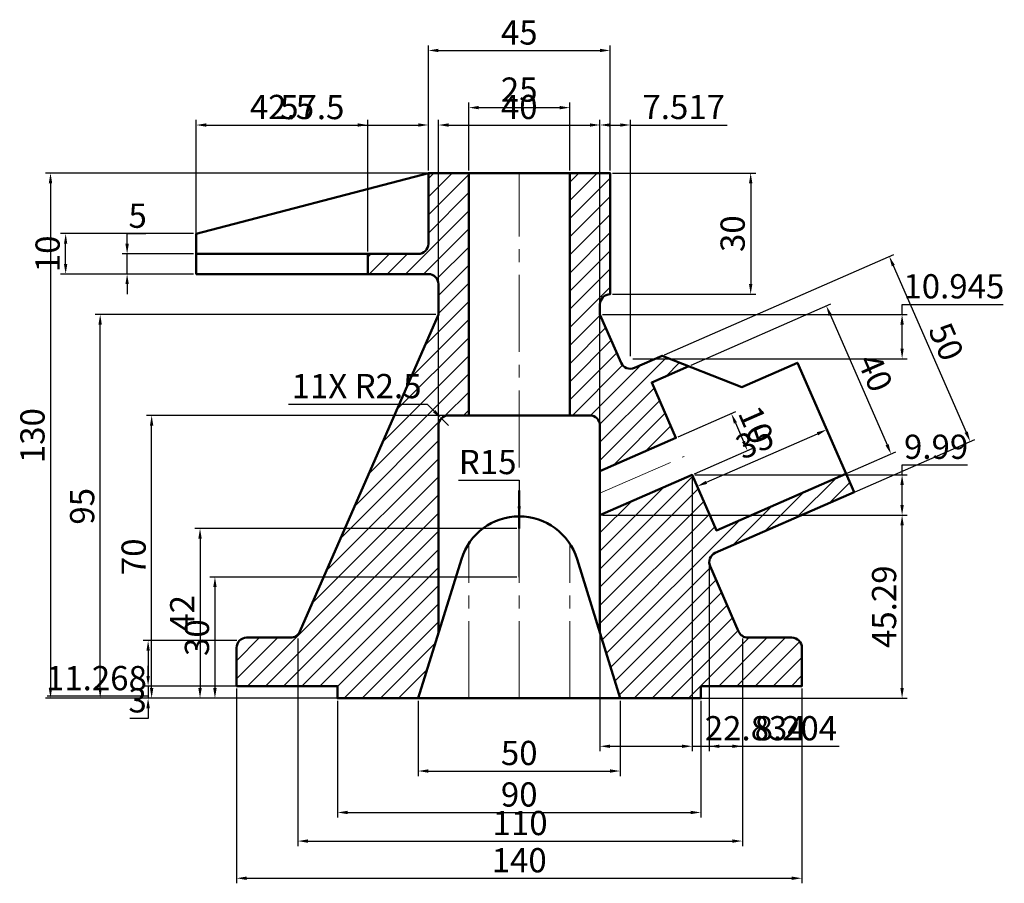
# Model space of a CAD drawing. Units: millimetres. Extents: x 76 to 320, y 39 to 253.
import ezdxf

# ---------------------------------------------------------------- set-up
doc = ezdxf.new("R2010")
doc.units = ezdxf.units.MM
doc.linetypes.add('CENTER2', pattern=[28.575, 19.05, -3.175, 3.175, -3.175])
for name, color, linetype, lineweight in [('M-CNTR', 4, 'CENTER2', 18), ('M-DIMS', 2, 'Continuous', 25), ('M-HATC', 8, 'Continuous', 18), ('M-OUTL', 7, 'Continuous', 50)]:
    doc.layers.add(name, color=color, linetype=linetype, lineweight=lineweight)
doc.styles.get("Standard").update_dxf_attribs({"font": 'arial.ttf'})
doc.dimstyles.new('ISO-25', dxfattribs={"dimtxt": 6, "dimasz": 2.5, "dimexe": 1.25, "dimexo": 0.625, "dimtad": 1, "dimtoh": 1, "dimdec": 0, "dimtxsty": 'Standard', "dimcen": 2.5, "dimadec": 0, "dimazin": 0, "dimtfac": 1, "dimtdec": 0, "dimtmove": 0, "dimatfit": 3, "dimfxl": 1, "dimarcsym": 0})

# ---------------------------------------------------------------- blocks, each defined once
blk = doc.blocks.new('*D1')
at = {"layer": 'Defpoints', "color": 0, "transparency": 16777216}
for p in [(235.21, 169.38), (311.5, 148.18), (255.25, 123.57)]:
    blk.add_point(p, dxfattribs=at)
at = {"layer": 'M-DIMS', "color": 0, "lineweight": -2, "transparency": 16777216}
for p, q in [((235.78, 169.63), (292.6, 194.49)), ((292.46, 191.7), (310.5, 150.47)), ((255.82, 123.82), (312.64, 148.68))]:
    blk.add_line(p, q, dxfattribs=at)
at = {"layer": 'M-DIMS', "color": 0, "transparency": 16777216}
for points in [[(292.84, 191.86), (292.08, 191.53), (291.46, 193.99)], [(310.88, 150.64), (310.11, 150.3), (311.5, 148.18)]]:
    blk.add_solid(points, dxfattribs=at)
at = {"layer": 'M-DIMS', "color": 0, "transparency": 16777216, "insert": (304.86, 172.56), "char_height": 6, "attachment_point": 5, "rotation": 293.6294}
blk.add_mtext('50', dxfattribs=at)
blk = doc.blocks.new('*D2')
at = {"layer": 'Defpoints', "color": 0, "transparency": 16777216}
for p in [(241.8, 166.8), (291.91, 145.07), (257.83, 130.16)]:
    blk.add_point(p, dxfattribs=at)
at = {"layer": 'M-DIMS', "color": 0, "lineweight": -2, "transparency": 16777216}
for p, q in [((242.37, 167.05), (277.02, 182.21)), ((276.88, 179.42), (290.91, 147.36)), ((258.4, 130.41), (293.05, 145.57))]:
    blk.add_line(p, q, dxfattribs=at)
at = {"layer": 'M-DIMS', "color": 0, "transparency": 16777216}
for points in [[(277.26, 179.59), (276.5, 179.25), (275.88, 181.71)], [(291.29, 147.52), (290.52, 147.19), (291.91, 145.07)]]:
    blk.add_solid(points, dxfattribs=at)
at = {"layer": 'M-DIMS', "color": 0, "transparency": 16777216, "insert": (287.27, 164.87), "char_height": 6, "attachment_point": 5, "rotation": 293.6294}
blk.add_mtext('40', dxfattribs=at)
blk = doc.blocks.new('*D3')
at = {"layer": 'Defpoints', "color": 0, "transparency": 16777216}
for p in [(238.65, 149.05), (256.36, 145.89), (242.65, 139.89)]:
    blk.add_point(p, dxfattribs=at)
at = {"layer": 'M-DIMS', "color": 0, "lineweight": -2, "transparency": 16777216}
for p, q in [((239.22, 149.3), (253.5, 155.55)), ((253.36, 152.76), (255.36, 148.18)), ((243.23, 140.14), (257.51, 146.39))]:
    blk.add_line(p, q, dxfattribs=at)
at = {"layer": 'M-DIMS', "color": 0, "transparency": 16777216}
for points in [[(253.74, 152.93), (252.98, 152.59), (252.36, 155.05)], [(255.74, 148.34), (254.98, 148.01), (256.36, 145.89)]]:
    blk.add_solid(points, dxfattribs=at)
at = {"layer": 'M-DIMS', "color": 0, "transparency": 16777216, "insert": (257.74, 151.95), "char_height": 6, "attachment_point": 5, "rotation": 293.6294}
blk.add_mtext('10', dxfattribs=at)
blk = doc.blocks.new('*D4')
at = {"layer": 'Defpoints', "color": 0, "transparency": 16777216}
for p in [(199.82, 214.61), (83.75, 84.61), (199.82, 84.61)]:
    blk.add_point(p, dxfattribs=at)
at = {"layer": 'M-DIMS', "color": 0, "lineweight": -2, "transparency": 16777216}
for p, q in [((199.2, 214.61), (82.5, 214.61)), ((83.75, 212.11), (83.75, 87.11)), ((199.2, 84.61), (82.5, 84.61))]:
    blk.add_line(p, q, dxfattribs=at)
at = {"layer": 'M-DIMS', "color": 0, "transparency": 16777216}
for points in [[(83.33, 212.11), (84.16, 212.11), (83.75, 214.61)], [(83.33, 87.11), (84.16, 87.11), (83.75, 84.61)]]:
    blk.add_solid(points, dxfattribs=at)
at = {"layer": 'M-DIMS', "color": 0, "transparency": 16777216, "insert": (80.06, 149.61), "char_height": 6, "attachment_point": 5, "rotation": 90}
blk.add_mtext('130', dxfattribs=at)
blk = doc.blocks.new('*D5')
at = {"layer": 'Defpoints', "color": 0, "transparency": 16777216}
for p in [(222.32, 214.61), (222.32, 184.61), (257.14, 184.61)]:
    blk.add_point(p, dxfattribs=at)
at = {"layer": 'M-DIMS', "color": 0, "lineweight": -2, "transparency": 16777216}
for p, q in [((222.95, 214.61), (258.39, 214.61)), ((257.14, 212.11), (257.14, 187.11)), ((222.95, 184.61), (258.39, 184.61))]:
    blk.add_line(p, q, dxfattribs=at)
at = {"layer": 'M-DIMS', "color": 0, "transparency": 16777216}
for points in [[(256.73, 212.11), (257.56, 212.11), (257.14, 214.61)], [(256.73, 187.11), (257.56, 187.11), (257.14, 184.61)]]:
    blk.add_solid(points, dxfattribs=at)
at = {"layer": 'M-DIMS', "color": 0, "transparency": 16777216, "insert": (253.45, 199.61), "char_height": 6, "attachment_point": 5, "rotation": 90}
blk.add_mtext('30', dxfattribs=at)
blk = doc.blocks.new('*D6')
at = {"layer": 'Defpoints', "color": 0, "transparency": 16777216}
for p in [(96.05, 179.61), (179.82, 179.61), (199.82, 84.61)]:
    blk.add_point(p, dxfattribs=at)
at = {"layer": 'M-DIMS', "color": 0, "lineweight": -2, "transparency": 16777216}
for p, q in [((179.2, 179.61), (94.8, 179.61)), ((96.05, 87.11), (96.05, 177.11)), ((199.2, 84.61), (94.8, 84.61))]:
    blk.add_line(p, q, dxfattribs=at)
at = {"layer": 'M-DIMS', "color": 0, "transparency": 16777216}
for points in [[(95.63, 177.11), (96.46, 177.11), (96.05, 179.61)], [(95.63, 87.11), (96.46, 87.11), (96.05, 84.61)]]:
    blk.add_solid(points, dxfattribs=at)
at = {"layer": 'M-DIMS', "color": 0, "transparency": 16777216, "insert": (92.36, 132.11), "char_height": 6, "attachment_point": 5, "rotation": 90}
blk.add_mtext('95', dxfattribs=at)
blk = doc.blocks.new('*D7')
at = {"layer": 'Defpoints', "color": 0, "transparency": 16777216}
for p in [(108.8, 154.61), (199.82, 154.61), (199.82, 84.61)]:
    blk.add_point(p, dxfattribs=at)
at = {"layer": 'M-DIMS', "color": 0, "lineweight": -2, "transparency": 16777216}
for p, q in [((199.2, 154.61), (107.55, 154.61)), ((108.8, 87.11), (108.8, 152.11)), ((199.2, 84.61), (107.55, 84.61))]:
    blk.add_line(p, q, dxfattribs=at)
at = {"layer": 'M-DIMS', "color": 0, "transparency": 16777216}
for points in [[(108.38, 152.11), (109.21, 152.11), (108.8, 154.61)], [(108.38, 87.11), (109.21, 87.11), (108.8, 84.61)]]:
    blk.add_solid(points, dxfattribs=at)
at = {"layer": 'M-DIMS', "color": 0, "transparency": 16777216, "insert": (105.11, 119.61), "char_height": 6, "attachment_point": 5, "rotation": 90}
blk.add_mtext('70', dxfattribs=at)
blk = doc.blocks.new('*D8')
at = {"layer": 'Defpoints', "color": 0, "transparency": 16777216}
for p in [(222.32, 244.97), (177.32, 214.61), (222.32, 214.61)]:
    blk.add_point(p, dxfattribs=at)
at = {"layer": 'M-DIMS', "color": 0, "lineweight": -2, "transparency": 16777216}
for p, q in [((177.32, 215.23), (177.32, 246.22)), ((179.82, 244.97), (219.82, 244.97)), ((222.32, 215.23), (222.32, 246.22))]:
    blk.add_line(p, q, dxfattribs=at)
at = {"layer": 'M-DIMS', "color": 0, "transparency": 16777216}
for points in [[(179.82, 245.38), (179.82, 244.55), (177.32, 244.97)], [(219.82, 245.38), (219.82, 244.55), (222.32, 244.97)]]:
    blk.add_solid(points, dxfattribs=at)
at = {"layer": 'M-DIMS', "color": 0, "transparency": 16777216, "insert": (199.82, 248.64), "char_height": 6, "attachment_point": 5}
blk.add_mtext('45', dxfattribs=at)
blk = doc.blocks.new('*D9')
at = {"layer": 'Defpoints', "color": 0, "transparency": 16777216}
for p in [(212.32, 230.81), (187.32, 214.61), (212.32, 214.61)]:
    blk.add_point(p, dxfattribs=at)
at = {"layer": 'M-DIMS', "color": 0, "lineweight": -2, "transparency": 16777216}
for p, q in [((187.32, 215.23), (187.32, 232.06)), ((212.32, 215.23), (212.32, 232.06)), ((189.82, 230.81), (209.82, 230.81))]:
    blk.add_line(p, q, dxfattribs=at)
at = {"layer": 'M-DIMS', "color": 0, "transparency": 16777216}
for points in [[(189.82, 231.23), (189.82, 230.39), (187.32, 230.81)], [(209.82, 231.23), (209.82, 230.39), (212.32, 230.81)]]:
    blk.add_solid(points, dxfattribs=at)
at = {"layer": 'M-DIMS', "color": 0, "transparency": 16777216, "insert": (199.82, 234.5), "char_height": 6, "attachment_point": 5}
blk.add_mtext('25', dxfattribs=at)
blk = doc.blocks.new('*D10')
at = {"layer": 'Defpoints', "color": 0, "transparency": 16777216}
for p in [(87.5, 199.61), (119.82, 199.61), (119.82, 189.61)]:
    blk.add_point(p, dxfattribs=at)
at = {"layer": 'M-DIMS', "color": 0, "lineweight": -2, "transparency": 16777216}
for p, q in [((119.2, 199.61), (86.25, 199.61)), ((87.5, 192.11), (87.5, 197.11)), ((119.2, 189.61), (86.25, 189.61))]:
    blk.add_line(p, q, dxfattribs=at)
at = {"layer": 'M-DIMS', "color": 0, "transparency": 16777216}
for points in [[(87.08, 197.11), (87.91, 197.11), (87.5, 199.61)], [(87.08, 192.11), (87.91, 192.11), (87.5, 189.61)]]:
    blk.add_solid(points, dxfattribs=at)
at = {"layer": 'M-DIMS', "color": 0, "transparency": 16777216, "insert": (83.81, 194.61), "char_height": 6, "attachment_point": 5, "rotation": 90}
blk.add_mtext('10', dxfattribs=at)
blk = doc.blocks.new('*D11')
at = {"layer": 'Defpoints', "color": 0, "transparency": 16777216}
for p in [(102.72, 194.61), (119.82, 194.61), (119.82, 189.61)]:
    blk.add_point(p, dxfattribs=at)
at = {"layer": 'M-DIMS', "color": 0, "lineweight": -2, "transparency": 16777216}
for p, q in [((102.72, 197.11), (102.72, 199.61)), ((102.72, 199.61), (107.32, 199.61)), ((119.2, 194.61), (101.47, 194.61)), ((102.72, 189.61), (102.72, 194.61)), ((119.2, 189.61), (101.47, 189.61)), ((102.72, 187.11), (102.72, 184.61))]:
    blk.add_line(p, q, dxfattribs=at)
at = {"layer": 'M-DIMS', "color": 0, "transparency": 16777216}
for points in [[(102.3, 197.11), (103.14, 197.11), (102.72, 194.61)], [(102.3, 187.11), (103.14, 187.11), (102.72, 189.61)]]:
    blk.add_solid(points, dxfattribs=at)
at = {"layer": 'M-DIMS', "color": 0, "transparency": 16777216, "insert": (105.33, 203.28), "char_height": 6, "attachment_point": 5}
blk.add_mtext('5', dxfattribs=at)
blk = doc.blocks.new('*D12')
at = {"layer": 'Defpoints', "color": 0, "transparency": 16777216}
for p in [(129.82, 87.61), (269.82, 87.61), (269.82, 40.03)]:
    blk.add_point(p, dxfattribs=at)
at = {"layer": 'M-DIMS', "color": 0, "lineweight": -2, "transparency": 16777216}
for p, q in [((129.82, 86.98), (129.82, 38.78)), ((269.82, 86.98), (269.82, 38.78)), ((132.32, 40.03), (267.32, 40.03))]:
    blk.add_line(p, q, dxfattribs=at)
at = {"layer": 'M-DIMS', "color": 0, "transparency": 16777216}
for points in [[(132.32, 40.45), (132.32, 39.62), (129.82, 40.03)], [(267.32, 40.45), (267.32, 39.62), (269.82, 40.03)]]:
    blk.add_solid(points, dxfattribs=at)
at = {"layer": 'M-DIMS', "color": 0, "transparency": 16777216, "insert": (199.82, 43.72), "char_height": 6, "attachment_point": 5}
blk.add_mtext('140', dxfattribs=at)
blk = doc.blocks.new('*D13')
at = {"layer": 'Defpoints', "color": 0, "transparency": 16777216}
for p in [(174.82, 84.61), (224.82, 84.61), (224.82, 66.58)]:
    blk.add_point(p, dxfattribs=at)
at = {"layer": 'M-DIMS', "color": 0, "lineweight": -2, "transparency": 16777216}
for p, q in [((174.82, 83.98), (174.82, 65.33)), ((224.82, 83.98), (224.82, 65.33)), ((177.32, 66.58), (222.32, 66.58))]:
    blk.add_line(p, q, dxfattribs=at)
at = {"layer": 'M-DIMS', "color": 0, "transparency": 16777216}
for points in [[(177.32, 67), (177.32, 66.16), (174.82, 66.58)], [(222.32, 67), (222.32, 66.16), (224.82, 66.58)]]:
    blk.add_solid(points, dxfattribs=at)
at = {"layer": 'M-DIMS', "color": 0, "transparency": 16777216, "insert": (199.82, 70.27), "char_height": 6, "attachment_point": 5}
blk.add_mtext('50', dxfattribs=at)
blk = doc.blocks.new('*D14')
at = {"layer": 'Defpoints', "color": 0, "transparency": 16777216}
for p in [(154.82, 84.61), (244.82, 84.61), (244.82, 56.32)]:
    blk.add_point(p, dxfattribs=at)
at = {"layer": 'M-DIMS', "color": 0, "lineweight": -2, "transparency": 16777216}
for p, q in [((154.82, 83.98), (154.82, 55.07)), ((244.82, 83.98), (244.82, 55.07)), ((157.32, 56.32), (242.32, 56.32))]:
    blk.add_line(p, q, dxfattribs=at)
at = {"layer": 'M-DIMS', "color": 0, "transparency": 16777216}
for points in [[(157.32, 56.73), (157.32, 55.9), (154.82, 56.32)], [(242.32, 56.73), (242.32, 55.9), (244.82, 56.32)]]:
    blk.add_solid(points, dxfattribs=at)
at = {"layer": 'M-DIMS', "color": 0, "transparency": 16777216, "insert": (199.82, 60), "char_height": 6, "attachment_point": 5}
blk.add_mtext('90', dxfattribs=at)
blk = doc.blocks.new('*D15')
at = {"layer": 'Defpoints', "color": 0, "transparency": 16777216}
for p in [(144.99, 99.99), (255.09, 100.01), (255.09, 49.24)]:
    blk.add_point(p, dxfattribs=at)
at = {"layer": 'M-DIMS', "color": 0, "lineweight": -2, "transparency": 16777216}
for p, q in [((144.99, 99.37), (144.99, 47.99)), ((255.09, 99.39), (255.09, 47.99)), ((147.49, 49.24), (252.59, 49.24))]:
    blk.add_line(p, q, dxfattribs=at)
at = {"layer": 'M-DIMS', "color": 0, "transparency": 16777216}
for points in [[(147.49, 49.65), (147.49, 48.82), (144.99, 49.24)], [(252.59, 49.65), (252.59, 48.82), (255.09, 49.24)]]:
    blk.add_solid(points, dxfattribs=at)
at = {"layer": 'M-DIMS', "color": 0, "transparency": 16777216, "insert": (200.04, 52.93), "char_height": 6, "attachment_point": 5}
blk.add_mtext('110', dxfattribs=at)
blk = doc.blocks.new('*D16')
at = {"layer": 'Defpoints', "color": 0, "transparency": 16777216}
for p in [(199.82, 114.61), (124.47, 84.61), (199.82, 84.61)]:
    blk.add_point(p, dxfattribs=at)
at = {"layer": 'M-DIMS', "color": 0, "lineweight": -2, "transparency": 16777216}
for p, q in [((199.2, 114.61), (123.22, 114.61)), ((124.47, 112.11), (124.47, 87.11)), ((199.2, 84.61), (123.22, 84.61))]:
    blk.add_line(p, q, dxfattribs=at)
at = {"layer": 'M-DIMS', "color": 0, "transparency": 16777216}
for points in [[(124.05, 112.11), (124.89, 112.11), (124.47, 114.61)], [(124.05, 87.11), (124.89, 87.11), (124.47, 84.61)]]:
    blk.add_solid(points, dxfattribs=at)
at = {"layer": 'M-DIMS', "color": 0, "transparency": 16777216, "insert": (120.78, 99.61), "char_height": 6, "attachment_point": 5, "rotation": 90}
blk.add_mtext('30', dxfattribs=at)
blk = doc.blocks.new('*D17')
at = {"layer": 'Defpoints', "color": 0, "transparency": 16777216}
for p in [(199.82, 126.61), (120.78, 84.61), (199.82, 84.61)]:
    blk.add_point(p, dxfattribs=at)
at = {"layer": 'M-DIMS', "color": 0, "lineweight": -2, "transparency": 16777216}
for p, q in [((199.2, 126.61), (119.53, 126.61)), ((120.78, 124.11), (120.78, 87.11)), ((199.2, 84.61), (119.53, 84.61))]:
    blk.add_line(p, q, dxfattribs=at)
at = {"layer": 'M-DIMS', "color": 0, "transparency": 16777216}
for points in [[(120.36, 124.11), (121.2, 124.11), (120.78, 126.61)], [(120.36, 87.11), (121.2, 87.11), (120.78, 84.61)]]:
    blk.add_solid(points, dxfattribs=at)
at = {"layer": 'M-DIMS', "color": 0, "transparency": 16777216, "insert": (117.14, 105.61), "char_height": 6, "attachment_point": 5, "rotation": 90}
blk.add_mtext('42', dxfattribs=at)
blk = doc.blocks.new('*D18')
at = {"layer": 'Defpoints', "color": 0, "transparency": 16777216}
for p in [(177.32, 226.51), (177.32, 214.61), (119.82, 199.61)]:
    blk.add_point(p, dxfattribs=at)
at = {"layer": 'M-DIMS', "color": 0, "lineweight": -2, "transparency": 16777216}
for p, q in [((119.82, 200.23), (119.82, 227.76)), ((177.32, 215.23), (177.32, 227.76)), ((122.32, 226.51), (174.82, 226.51))]:
    blk.add_line(p, q, dxfattribs=at)
at = {"layer": 'M-DIMS', "color": 0, "transparency": 16777216}
for points in [[(122.32, 226.92), (122.32, 226.09), (119.82, 226.51)], [(174.82, 226.92), (174.82, 226.09), (177.32, 226.51)]]:
    blk.add_solid(points, dxfattribs=at)
at = {"layer": 'M-DIMS', "color": 0, "transparency": 16777216, "insert": (148.57, 230.18), "char_height": 6, "attachment_point": 5}
blk.add_mtext('57.5', dxfattribs=at)
blk = doc.blocks.new('*D19')
at = {"layer": 'Defpoints', "color": 0, "transparency": 16777216}
for p in [(162.32, 226.51), (162.32, 194.61), (119.82, 189.61)]:
    blk.add_point(p, dxfattribs=at)
at = {"layer": 'M-DIMS', "color": 0, "lineweight": -2, "transparency": 16777216}
for p, q in [((119.82, 190.23), (119.82, 227.76)), ((162.32, 195.23), (162.32, 227.76)), ((122.32, 226.51), (159.82, 226.51))]:
    blk.add_line(p, q, dxfattribs=at)
at = {"layer": 'M-DIMS', "color": 0, "transparency": 16777216}
for points in [[(122.32, 226.92), (122.32, 226.09), (119.82, 226.51)], [(159.82, 226.92), (159.82, 226.09), (162.32, 226.51)]]:
    blk.add_solid(points, dxfattribs=at)
at = {"layer": 'M-DIMS', "color": 0, "transparency": 16777216, "insert": (141.07, 230.2), "char_height": 6, "attachment_point": 5}
blk.add_mtext('42.5', dxfattribs=at)
blk = doc.blocks.new('*D20')
at = {"layer": 'Defpoints', "color": 0, "transparency": 16777216}
for p in [(130.55, 98.87), (107.92, 87.61), (129.82, 87.61)]:
    blk.add_point(p, dxfattribs=at)
at = {"layer": 'M-DIMS', "color": 0, "lineweight": -2, "transparency": 16777216}
for p, q in [((129.93, 98.87), (106.67, 98.87)), ((107.92, 96.37), (107.92, 90.11)), ((129.2, 87.61), (106.67, 87.61)), ((107.92, 87.61), (107.92, 85.11)), ((107.92, 85.11), (82.94, 85.11))]:
    blk.add_line(p, q, dxfattribs=at)
at = {"layer": 'M-DIMS', "color": 0, "transparency": 16777216}
for points in [[(107.5, 96.37), (108.34, 96.37), (107.92, 98.87)], [(107.5, 90.11), (108.34, 90.11), (107.92, 87.61)]]:
    blk.add_solid(points, dxfattribs=at)
at = {"layer": 'M-DIMS', "color": 0, "transparency": 16777216, "insert": (95.12, 88.8), "char_height": 6, "attachment_point": 5}
blk.add_mtext('11.268', dxfattribs=at)
blk = doc.blocks.new('*D21')
at = {"layer": 'Defpoints', "color": 0, "transparency": 16777216}
for p in [(154.82, 87.61), (107.92, 84.61), (154.82, 84.61)]:
    blk.add_point(p, dxfattribs=at)
at = {"layer": 'M-DIMS', "color": 0, "lineweight": -2, "transparency": 16777216}
for p, q in [((107.92, 90.11), (107.92, 92.61)), ((154.2, 87.61), (106.67, 87.61)), ((107.92, 87.61), (107.92, 84.61)), ((154.2, 84.61), (106.67, 84.61)), ((107.92, 82.11), (107.92, 79.61)), ((107.92, 79.61), (103.37, 79.61))]:
    blk.add_line(p, q, dxfattribs=at)
at = {"layer": 'M-DIMS', "color": 0, "transparency": 16777216}
for points in [[(107.5, 90.11), (108.34, 90.11), (107.92, 87.61)], [(107.5, 82.11), (108.34, 82.11), (107.92, 84.61)]]:
    blk.add_solid(points, dxfattribs=at)
at = {"layer": 'M-DIMS', "color": 0, "transparency": 16777216, "insert": (105.33, 83.3), "char_height": 6, "attachment_point": 5}
blk.add_mtext('3', dxfattribs=at)
blk = doc.blocks.new('*D22')
at = {"layer": 'Defpoints', "color": 0, "transparency": 16777216}
for p in [(219.82, 226.51), (179.82, 152.11), (219.82, 152.11)]:
    blk.add_point(p, dxfattribs=at)
at = {"layer": 'M-DIMS', "color": 0, "lineweight": -2, "transparency": 16777216}
for p, q in [((179.82, 152.73), (179.82, 227.76)), ((219.82, 152.73), (219.82, 227.76)), ((182.32, 226.51), (217.32, 226.51))]:
    blk.add_line(p, q, dxfattribs=at)
at = {"layer": 'M-DIMS', "color": 0, "transparency": 16777216}
for points in [[(182.32, 226.92), (182.32, 226.09), (179.82, 226.51)], [(217.32, 226.92), (217.32, 226.09), (219.82, 226.51)]]:
    blk.add_solid(points, dxfattribs=at)
at = {"layer": 'M-DIMS', "color": 0, "transparency": 16777216, "insert": (199.82, 230.2), "char_height": 6, "attachment_point": 5}
blk.add_mtext('40', dxfattribs=at)
blk = doc.blocks.new('*D23')
at = {"layer": 'Defpoints', "color": 0, "transparency": 16777216}
for p in [(227.34, 226.51), (219.82, 179.61), (227.34, 168.66)]:
    blk.add_point(p, dxfattribs=at)
at = {"layer": 'M-DIMS', "color": 0, "lineweight": -2, "transparency": 16777216}
for p, q in [((219.82, 180.23), (219.82, 227.76)), ((227.34, 169.29), (227.34, 227.76)), ((222.32, 226.51), (224.84, 226.51)), ((227.34, 226.51), (251.29, 226.51))]:
    blk.add_line(p, q, dxfattribs=at)
at = {"layer": 'M-DIMS', "color": 0, "transparency": 16777216}
for points in [[(222.32, 226.92), (222.32, 226.09), (219.82, 226.51)], [(224.84, 226.92), (224.84, 226.09), (227.34, 226.51)]]:
    blk.add_solid(points, dxfattribs=at)
at = {"layer": 'M-DIMS', "color": 0, "transparency": 16777216, "insert": (240.56, 230.2), "char_height": 6, "attachment_point": 5}
blk.add_mtext('7.517', dxfattribs=at)
blk = doc.blocks.new('*D24')
at = {"layer": 'Defpoints', "color": 0, "transparency": 16777216}
for p in [(219.82, 179.61), (294.64, 179.61), (227.34, 168.66)]:
    blk.add_point(p, dxfattribs=at)
at = {"layer": 'M-DIMS', "color": 0, "lineweight": -2, "transparency": 16777216}
for p, q in [((294.64, 179.61), (294.64, 182.11)), ((294.64, 182.11), (319.65, 182.11)), ((220.45, 179.61), (295.89, 179.61)), ((294.64, 171.16), (294.64, 177.11)), ((227.96, 168.66), (295.89, 168.66))]:
    blk.add_line(p, q, dxfattribs=at)
at = {"layer": 'M-DIMS', "color": 0, "transparency": 16777216}
for points in [[(294.22, 177.11), (295.05, 177.11), (294.64, 179.61)], [(294.22, 171.16), (295.05, 171.16), (294.64, 168.66)]]:
    blk.add_solid(points, dxfattribs=at)
at = {"layer": 'M-DIMS', "color": 0, "transparency": 16777216, "insert": (307.46, 185.8), "char_height": 6, "attachment_point": 5}
blk.add_mtext('10.945', dxfattribs=at)
blk = doc.blocks.new('*D25')
at = {"layer": 'Defpoints', "color": 0, "transparency": 16777216}
for p in [(242.65, 139.89), (219.82, 129.9), (242.65, 72.71)]:
    blk.add_point(p, dxfattribs=at)
at = {"layer": 'M-DIMS', "color": 0, "lineweight": -2, "transparency": 16777216}
for p, q in [((242.65, 139.26), (242.65, 71.46)), ((219.82, 129.27), (219.82, 71.46)), ((222.32, 72.71), (240.15, 72.71)), ((242.65, 72.71), (271.39, 72.71))]:
    blk.add_line(p, q, dxfattribs=at)
at = {"layer": 'M-DIMS', "color": 0, "transparency": 16777216}
for points in [[(222.32, 73.12), (222.32, 72.29), (219.82, 72.71)], [(240.15, 73.12), (240.15, 72.29), (242.65, 72.71)]]:
    blk.add_solid(points, dxfattribs=at)
at = {"layer": 'M-DIMS', "color": 0, "transparency": 16777216, "insert": (258.27, 76.4), "char_height": 6, "attachment_point": 5}
blk.add_mtext('22.834', dxfattribs=at)
blk = doc.blocks.new('*D26')
at = {"layer": 'Defpoints', "color": 0, "transparency": 16777216}
for p in [(242.65, 139.89), (294.64, 139.89), (219.82, 129.9)]:
    blk.add_point(p, dxfattribs=at)
at = {"layer": 'M-DIMS', "color": 0, "lineweight": -2, "transparency": 16777216}
for p, q in [((294.64, 139.89), (294.64, 142.39)), ((294.64, 142.39), (310.86, 142.39)), ((243.28, 139.89), (295.89, 139.89)), ((294.64, 132.4), (294.64, 137.39)), ((220.45, 129.9), (295.89, 129.9))]:
    blk.add_line(p, q, dxfattribs=at)
at = {"layer": 'M-DIMS', "color": 0, "transparency": 16777216}
for points in [[(294.22, 137.39), (295.05, 137.39), (294.64, 139.89)], [(294.22, 132.4), (295.05, 132.4), (294.64, 129.9)]]:
    blk.add_solid(points, dxfattribs=at)
at = {"layer": 'M-DIMS', "color": 0, "transparency": 16777216, "insert": (303.06, 146.08), "char_height": 6, "attachment_point": 5}
blk.add_mtext('9.99', dxfattribs=at)
blk = doc.blocks.new('*D27')
at = {"layer": 'Defpoints', "color": 0, "transparency": 16777216}
for p in [(219.82, 129.9), (294.64, 129.9), (224.82, 84.61)]:
    blk.add_point(p, dxfattribs=at)
at = {"layer": 'M-DIMS', "color": 0, "lineweight": -2, "transparency": 16777216}
for p, q in [((220.45, 129.9), (295.89, 129.9)), ((294.64, 87.11), (294.64, 127.4)), ((225.45, 84.61), (295.89, 84.61))]:
    blk.add_line(p, q, dxfattribs=at)
at = {"layer": 'M-DIMS', "color": 0, "transparency": 16777216}
for points in [[(294.22, 127.4), (295.05, 127.4), (294.64, 129.9)], [(294.22, 87.11), (295.05, 87.11), (294.64, 84.61)]]:
    blk.add_solid(points, dxfattribs=at)
at = {"layer": 'M-DIMS', "color": 0, "transparency": 16777216, "insert": (290.95, 107.25), "char_height": 6, "attachment_point": 5, "rotation": 90}
blk.add_mtext('45.29', dxfattribs=at)
blk = doc.blocks.new('*D28')
at = {"layer": 'Defpoints', "color": 0, "transparency": 16777216}
for p in [(246.88, 118.22), (255.09, 100.01), (255.09, 72.71)]:
    blk.add_point(p, dxfattribs=at)
at = {"layer": 'M-DIMS', "color": 0, "lineweight": -2, "transparency": 16777216}
for p, q in [((246.88, 117.6), (246.88, 71.46)), ((255.09, 99.39), (255.09, 71.46)), ((249.38, 72.71), (252.59, 72.71)), ((255.09, 72.71), (279.07, 72.71))]:
    blk.add_line(p, q, dxfattribs=at)
at = {"layer": 'M-DIMS', "color": 0, "transparency": 16777216}
for points in [[(249.38, 73.12), (249.38, 72.29), (246.88, 72.71)], [(252.59, 73.12), (252.59, 72.29), (255.09, 72.71)]]:
    blk.add_solid(points, dxfattribs=at)
at = {"layer": 'M-DIMS', "color": 0, "transparency": 16777216, "insert": (268.33, 76.4), "char_height": 6, "attachment_point": 5}
blk.add_mtext('8.204', dxfattribs=at)
blk = doc.blocks.new('*D29')
at = {"layer": 'Defpoints', "color": 0, "transparency": 16777216}
for p in [(275.96, 151.08), (280.73, 140.18), (248.67, 126.15)]:
    blk.add_point(p, dxfattribs=at)
at = {"layer": 'M-DIMS', "color": 0, "lineweight": -2, "transparency": 16777216}
for p, q in [((280.48, 140.75), (275.46, 152.22)), ((246.19, 138.05), (273.67, 150.08)), ((248.42, 126.72), (243.4, 138.19))]:
    blk.add_line(p, q, dxfattribs=at)
at = {"layer": 'M-DIMS', "color": 0, "transparency": 16777216}
for points in [[(273.51, 150.46), (273.84, 149.69), (275.96, 151.08)], [(246.02, 138.43), (246.35, 137.67), (243.9, 137.05)]]:
    blk.add_solid(points, dxfattribs=at)
at = {"layer": 'M-DIMS', "color": 0, "transparency": 16777216, "insert": (258.45, 147.44), "char_height": 6, "attachment_point": 5, "rotation": 23.6294}
blk.add_mtext('35', dxfattribs=at)
blk = doc.blocks.new('*D30')
at = {"layer": 'Defpoints', "color": 0, "transparency": 16777216}
for p in [(199.82, 129.61), (199.82, 114.61)]:
    blk.add_point(p, dxfattribs=at)
at = {"layer": 'M-DIMS', "color": 0, "lineweight": -2, "transparency": 16777216}
for p, q in [((184.81, 138.61), (199.82, 138.61)), ((199.82, 138.61), (199.82, 132.11)), ((199.82, 114.61), (199.82, 129.61))]:
    blk.add_line(p, q, dxfattribs=at)
at = {"layer": 'M-DIMS', "color": 0, "transparency": 16777216}
blk.add_solid([(200.24, 132.11), (199.4, 132.11), (199.82, 129.61)], dxfattribs=at)
at = {"layer": 'M-DIMS', "color": 0, "transparency": 16777216, "insert": (192, 142.3), "char_height": 6, "attachment_point": 5}
blk.add_mtext('R15', dxfattribs=at)
blk = doc.blocks.new('*D31')
at = {"layer": 'Defpoints', "color": 0, "transparency": 16777216}
for p in [(180.55, 153.87), (182.32, 152.11)]:
    blk.add_point(p, dxfattribs=at)
at = {"layer": 'M-DIMS', "color": 0, "lineweight": -2, "transparency": 16777216}
for p, q in [((142.69, 157.41), (177.02, 157.41)), ((177.02, 157.41), (178.79, 155.64)), ((182.32, 152.11), (180.55, 153.87))]:
    blk.add_line(p, q, dxfattribs=at)
at = {"layer": 'M-DIMS', "color": 0, "transparency": 16777216}
blk.add_solid([(179.08, 155.94), (178.49, 155.35), (180.55, 153.87)], dxfattribs=at)
at = {"layer": 'M-DIMS', "color": 0, "transparency": 16777216, "insert": (159.54, 161.1), "char_height": 6, "attachment_point": 5}
blk.add_mtext('11X R2.5', dxfattribs=at)

msp = doc.modelspace()

# ---------------------------------------------------------------- hatches: boundary and pattern name
at = {"layer": 'M-HATC'}
h = msp.add_hatch(dxfattribs=at)
h.set_pattern_fill('ANSI31', color=256)
h.paths.add_polyline_path([(179.8208, 152.1071, -0.41421356), (182.3208, 154.6071), (187.3208, 154.6071), (187.3208, 214.6071), (177.3208, 214.6071), (177.3208, 197.1071, -0.41421356), (174.8208, 194.6071), (162.3208, 194.6071), (162.3208, 189.6071), (177.3208, 189.6071, -0.41421356), (179.8208, 187.1071), (179.8208, 179.6071), (145.4762, 101.1051, -0.29797338), (143.1858, 99.6071), (132.3208, 99.6071, 0.41421356), (129.8208, 97.1071), (129.8208, 87.6071), (154.8208, 87.6071), (154.8208, 84.6071), (174.8208, 84.6071), (179.8208, 100.7425)])
h.paths.add_polyline_path([(222.3208, 184.6071), (222.3208, 214.6071), (212.3208, 214.6071), (212.3208, 154.6071), (217.3208, 154.6071, -0.41421356), (219.8208, 152.1071), (219.8208, 140.8147), (238.6467, 149.051), (232.6344, 162.7934), (241.796, 166.8016), (235.2111, 169.3783), (228.3399, 166.3721, -0.41421356), (225.0475, 167.6605), (219.8208, 179.6071), (219.8208, 182.1071, -0.41421356)])
h = msp.add_hatch(dxfattribs=at)
h.set_pattern_fill('ANSI31', color=256)
h.paths.add_polyline_path([(247.0925, 117.2718, -0.41421356), (248.3808, 120.5643), (282.7367, 135.595), (280.7326, 140.1757), (248.6671, 126.1471), (242.6549, 139.8894), (219.8208, 129.8995), (219.8208, 100.7425), (224.8208, 84.6071), (244.8208, 84.6071), (244.8208, 87.6071), (269.8208, 87.6071), (269.8208, 97.1071, 0.41421356), (267.3208, 99.6071), (256.4558, 99.6071, -0.29797338), (254.1654, 101.1051)])

# ---------------------------------------------------------------- linework, layer by layer
at = {"layer": 'M-CNTR'}
for p, q in [((199.8208, 84.6071), (199.8208, 214.6071)), ((219.8208, 135.3571), (240.6508, 144.4702)), ((187.3208, 84.6071), (187.3208, 122.8987)), ((212.3208, 84.6071), (212.3208, 122.8987))]:
    msp.add_line(p, q, dxfattribs=at)
at = {"layer": 'M-OUTL'}
for p, q in [((187.3208, 154.6071), (187.3208, 214.6071)), ((212.3208, 154.6071), (212.3208, 214.6071)), ((162.3208, 194.6071), (162.3208, 189.6071)), ((199.8208, 126.6071), (199.8208, 136.0672))]:
    msp.add_line(p, q, dxfattribs=at)
for points in [[(224.8208, 84.6071), (244.8208, 84.6071), (244.8208, 87.6071), (269.8208, 87.6071), (269.8208, 97.1071, 0.41421356), (267.3208, 99.6071), (256.4558, 99.6071, -0.29797338), (254.1654, 101.1051), (247.0925, 117.2718, -0.41421356), (248.3808, 120.5643), (282.7367, 135.595), (268.7081, 167.6605), (254.9657, 161.6482), (235.2111, 169.3783), (228.3399, 166.3721, -0.41421356), (225.0475, 167.6605), (219.8208, 179.6071), (219.8208, 182.1071, -0.41421356), (222.3208, 184.6071), (222.3208, 184.6071), (222.3208, 214.6071), (199.8208, 214.6071), (177.3208, 214.6071), (119.8208, 199.6071), (119.8208, 194.6071)], [(177.3208, 214.6071), (177.3208, 197.1071, -0.41421356), (174.8208, 194.6071), (119.8208, 194.6071), (119.8208, 189.6071), (177.3208, 189.6071, -0.41421356), (179.8208, 187.1071), (179.8208, 179.6071), (145.4762, 101.1051, -0.29797338), (143.1858, 99.6071), (132.3208, 99.6071, 0.41421356), (129.8208, 97.1071), (129.8208, 87.6071), (154.8208, 87.6071), (154.8208, 84.6071), (174.8208, 84.6071)], [(219.8208, 100.7425), (219.8208, 152.1071, 0.41421356), (217.3208, 154.6071), (182.3208, 154.6071, 0.41421356), (179.8208, 152.1071), (179.8208, 100.7425)]]:
    msp.add_lwpolyline(points, format="xyb", dxfattribs=at)
for points in [[(219.8208, 140.8147), (238.6467, 149.051), (232.6344, 162.7934), (241.796, 166.8016)], [(219.8208, 129.8995), (242.6549, 139.8894), (248.6671, 126.1471), (280.7326, 140.1757)]]:
    msp.add_lwpolyline(points, dxfattribs=at)
msp.add_lwpolyline([(185.4929, 119.047), (174.8208, 84.6071), (224.8208, 84.6071), (214.1487, 119.047, 0.73703418)], format="xyb", close=True, dxfattribs=at)

# ---------------------------------------------------------------- dimensions: what is measured, and where the dimension line sits
at = {"layer": 'M-DIMS'}
for base, p1, p2, override, picture, middle in [((222.3208, 244.9667), (177.3208, 214.6071), (222.3208, 214.6071), {"dimclrd": 0, "dimclre": 0, "dimclrt": 0}, '*D8', (199.8208, 248.6429)), ((212.3208, 230.8091), (187.3208, 214.6071), (212.3208, 214.6071), {"dimclrd": 0, "dimclre": 0, "dimclrt": 0}, '*D9', (199.8208, 234.4975)), ((162.3208, 226.5071), (119.8208, 189.6071), (162.3208, 194.6071), {"dimdec": 1, "dimlfac": 1, "dimrnd": 0, "dimzin": 0, "dimdsep": 46, "dimlunit": 2}, '*D19', (141.0708, 230.1956)), ((177.3208, 226.5071), (119.8208, 199.6071), (177.3208, 214.6071), {"dimdec": 1, "dimlfac": 1, "dimrnd": 0, "dimzin": 0, "dimdsep": 46, "dimlunit": 2}, '*D18', (148.5708, 230.1833)), ((219.8208, 226.5071), (179.8208, 152.1071), (219.8208, 152.1071), {"dimdec": 0, "dimlfac": 1, "dimrnd": 0, "dimzin": 0, "dimdsep": 46, "dimlunit": 2}, '*D22', (199.8208, 230.1956)), ((227.3379, 226.5071), (219.8208, 179.6071), (227.3379, 168.6625), {"dimdec": 3, "dimlfac": 1, "dimrnd": 0, "dimzin": 0, "dimdsep": 46, "dimlunit": 2}, '*D23', (240.5618, 230.1956)), ((242.6549, 72.7071), (219.8208, 129.8995), (242.6549, 139.8894), {"dimdec": 3, "dimlfac": 1, "dimrnd": 0, "dimzin": 0, "dimdsep": 46, "dimlunit": 2}, '*D25', (258.273, 76.3976)), ((255.0875, 72.7071), (246.8834, 118.2246), (255.0875, 100.0149), {"dimdec": 3, "dimlfac": 1, "dimrnd": 0, "dimzin": 0, "dimdsep": 46, "dimlunit": 2}, '*D28', (268.3277, 76.3956)), ((255.0875, 49.2368), (144.9892, 99.992), (255.0875, 100.0149), {"dimclrd": 0, "dimclre": 0, "dimclrt": 0}, '*D15', (200.0383, 52.9253)), ((269.8208, 40.0343), (129.8208, 87.6071), (269.8208, 87.6071), {"dimclrd": 0, "dimclre": 0, "dimclrt": 0}, '*D12', (199.8208, 43.7228)), ((244.8208, 56.3157), (154.8208, 84.6071), (244.8208, 84.6071), {"dimclrd": 0, "dimclre": 0, "dimclrt": 0}, '*D14', (199.8208, 60.0041)), ((224.8208, 66.58), (174.8208, 84.6071), (224.8208, 84.6071), {"dimclrd": 0, "dimclre": 0, "dimclrt": 0}, '*D13', (199.8208, 70.2684))]:
    dim = msp.add_linear_dim(base=base, p1=p1, p2=p2, dimstyle='ISO-25', override=override, dxfattribs=at)
    dim.commit()
    dim.dimension.update_dxf_attribs({"geometry": picture, "text_midpoint": middle})
for base, p1, p2, angle, override, picture, middle in [((83.7456, 84.6071), (199.8208, 214.6071), (199.8208, 84.6071), 90, {"dimclrd": 0, "dimclre": 0, "dimclrt": 0}, '*D4', (80.0552, 149.6071)), ((257.144, 184.6071), (222.3208, 214.6071), (222.3208, 184.6071), 90, {"dimclrd": 0, "dimclre": 0, "dimclrt": 0}, '*D5', (253.4535, 199.6071)), ((102.7207, 194.6071), (119.8208, 189.6071), (119.8208, 194.6071), 90, {"dimclrd": 0, "dimclre": 0, "dimclrt": 0}, '*D11', (105.3348, 203.2833)), ((87.4956, 199.6071), (119.8208, 189.6071), (119.8208, 199.6071), 90, {"dimclrd": 0, "dimclre": 0, "dimclrt": 0}, '*D10', (83.8072, 194.6071)), ((294.6367, 179.6071), (227.3379, 168.6625), (219.8208, 179.6071), 90, {"dimdec": 3, "dimlfac": 1, "dimrnd": 0, "dimzin": 0, "dimdsep": 46, "dimlunit": 2}, '*D24', (307.4561, 185.7956)), ((96.0459, 179.6071), (199.8208, 84.6071), (179.8208, 179.6071), 90, {"dimclrd": 0, "dimclre": 0, "dimclrt": 0}, '*D6', (92.3574, 132.1071)), ((108.7981, 154.6071), (199.8208, 84.6071), (199.8208, 154.6071), 90, {"dimclrd": 0, "dimclre": 0, "dimclrt": 0}, '*D7', (105.1097, 119.6071)), ((275.9629, 151.078), (248.6671, 126.1471), (280.7326, 140.1757), 23.629378, {"dimdec": 0, "dimlfac": 1, "dimrnd": 0, "dimzin": 0, "dimdsep": 46, "dimlunit": 2}, '*D29', (258.4509, 147.4448)), ((294.6367, 139.8894), (219.8208, 129.8995), (242.6549, 139.8894), 90, {"dimdec": 2, "dimlfac": 1, "dimrnd": 0, "dimzin": 0, "dimdsep": 46, "dimlunit": 2}, '*D26', (303.0605, 146.0779)), ((294.6367, 129.8995), (224.8208, 84.6071), (219.8208, 129.8995), 90, {"dimdec": 2, "dimlfac": 1, "dimrnd": 0, "dimzin": 0, "dimdsep": 46, "dimlunit": 2}, '*D27', (290.9483, 107.2533)), ((120.7802, 84.6071), (199.8208, 126.6071), (199.8208, 84.6071), 90, {"dimclrd": 0, "dimclre": 0, "dimclrt": 0}, '*D17', (117.143, 105.6071)), ((124.4707, 84.6071), (199.8208, 114.6071), (199.8208, 84.6071), 90, {"dimclrd": 0, "dimclre": 0, "dimclrt": 0}, '*D16', (120.7802, 99.6071)), ((107.9208, 87.6071), (130.553, 98.8749), (129.8208, 87.6071), 90, {"dimdec": 3, "dimlfac": 1, "dimrnd": 0, "dimzin": 0, "dimdsep": 46, "dimlunit": 2}, '*D20', (95.1178, 88.7956)), ((107.9208, 84.6071), (154.8208, 87.6071), (154.8208, 84.6071), 90, {"dimdec": 0, "dimlfac": 1, "dimrnd": 0, "dimzin": 0, "dimdsep": 46, "dimlunit": 2}, '*D21', (105.3313, 83.2976))]:
    dim = msp.add_linear_dim(base=base, p1=p1, p2=p2, angle=angle, dimstyle='ISO-25', override=override, dxfattribs=at)
    dim.commit()
    dim.dimension.update_dxf_attribs({"geometry": picture, "text_midpoint": middle})
for p1, p2, distance, picture, middle in [((235.2111, 169.3783), (255.252, 123.5704), 61.3926, '*D1', (304.856, 172.56)), ((241.796, 166.8016), (257.8287, 130.1553), 37.1988, '*D2', (287.2715, 164.8668)), ((238.6467, 149.051), (242.6549, 139.8894), 14.9645, '*D3', (257.7398, 151.9467))]:
    dim = msp.add_aligned_dim(p1=p1, p2=p2, distance=distance, dimstyle='ISO-25', override={"dimclrd": 0, "dimclre": 0, "dimclrt": 0}, dxfattribs=at)
    dim.commit()
    dim.dimension.update_dxf_attribs({"geometry": picture, "text_midpoint": middle})
dim = msp.add_radius_dim(center=(182.3208, 152.1071), mpoint=(180.5531, 153.8749), text='11X <>', dimstyle='ISO-25', override={"dimdec": 1, "dimlfac": 1, "dimrnd": 0, "dimzin": 0, "dimdsep": 46, "dimlunit": 2}, dxfattribs=at)
dim.commit()
dim.dimension.update_dxf_attribs({"geometry": '*D31', "text_midpoint": (159.5427, 161.099)})
dim = msp.add_radius_dim(center=(199.8208, 114.6071), mpoint=(199.82, 129.6071), dimstyle='ISO-25', override={"dimdec": 0, "dimlfac": 1, "dimrnd": 0, "dimzin": 0, "dimdsep": 46, "dimlunit": 2}, dxfattribs=at)
dim.commit()
dim.dimension.update_dxf_attribs({"geometry": '*D30', "text_midpoint": (192.0035, 138.6071), "dimtype": 164})

doc.saveas('drawing.dxf')
